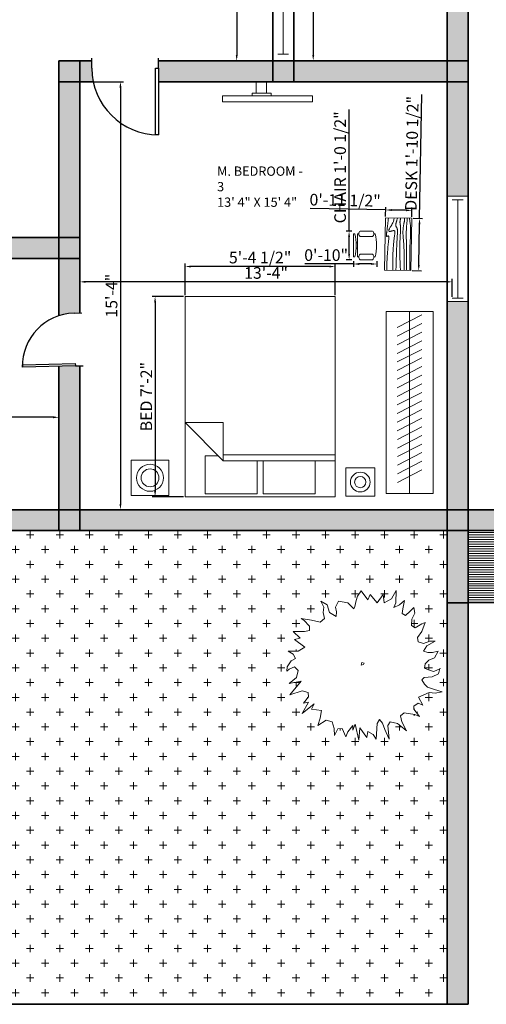
# Model space of a CAD drawing. Units: millimetres. Extents: x 2768 to 4359, y 795 to 1583.
# Tile 7 of 13: x 3880 to 4080, y 835 to 1258. Entities that reach past the tile are written whole.
import ezdxf

# ---------------------------------------------------------------- set-up
doc = ezdxf.new("R2010")
doc.units = ezdxf.units.MM
for name, color, linetype, lineweight in [('A-ANNO-DIMS', 90, 'Continuous', 18), ('A-AREA-IDEN', 190, 'Continuous', 18), ('A-DOOR-PATT', 251, 'Continuous', 13), ('A-EQPM', 50, 'Continuous', 18), ('A-FLOR-CASE', 50, 'Continuous', 18), ('A-FLOR-CASE-PATT', 50, 'Continuous', 13), ('A-WALL-PATT', 140, 'Continuous', 9), ('doors', 10, 'Continuous', 25), ('furniture', 50, 'Continuous', 18), ('GARDEN', 109, 'Continuous', 18), ('iron shutter', 251, 'Continuous', 18), ('L-PLNT-PATT', 109, 'Continuous', 13), ('walls', 140, 'Continuous', 35), ('windows', 30, 'Continuous', 18)]:
    doc.layers.add(name, color=color, linetype=linetype, lineweight=lineweight)
doc.styles.get("Standard").update_dxf_attribs({"font": 'arial.ttf'})
doc.dimstyles.new('ISO-25', dxfattribs={"dimtxt": 5, "dimasz": 2.5, "dimexe": 1.25, "dimexo": 0.625, "dimtad": 1, "dimdec": 0, "dimlunit": 3, "dimtxsty": 'Standard', "dimcen": 2.5, "dimadec": 0, "dimazin": 0, "dimtfac": 1, "dimtdec": 0, "dimtmove": 0, "dimatfit": 3, "dimfxl": 1, "dimarcsym": 0})

# ---------------------------------------------------------------- blocks, each defined once
blk = doc.blocks.new('*U2')
for p, q in [((0, 0), (0, -6)), ((40, 0), (40, -6))]:
    blk.add_line(p, q)
blk.add_lwpolyline([(0, 0), (0, 40), (1.75, 40), (1.75, 0)], close=True)
blk.add_arc((0, 0), 40, 0, 90)
blk = doc.blocks.new('*U39')
for p, q in [((0, 4), (0, 0)), ((36, 4), (36, 0)), ((0, 2), (36, 2))]:
    blk.add_line(p, q)
blk = doc.blocks.new('Bed - Queen')
for p, q in [((0, -80.00003), (0, 0)), ((0, 0), (59.99999, 0)), ((59.99999, 0), (59.99999, -80.00003)), ((7.99999, -1.2), (28.79998, -1.2)), ((7.99999, -14.4), (7.99999, -1.2)), ((28.79998, -1.2), (28.79998, -14.4)), ((31.19999, -1.2), (51.99999, -1.2)), ((31.19999, -14.4), (31.19999, -1.2)), ((51.99999, -1.2), (51.99999, -16.4)), ((0, -14.4), (44.8, -14.4)), ((59.99999, -29.6), (44.8, -14.4)), ((44.8, -14.4), (44.8, -29.6)), ((44.8, -16.8), (0, -16.8)), ((51.99999, -16.4), (46.79936, -16.4)), ((44.8, -29.6), (59.99999, -29.6)), ((59.99999, -80.00003), (0, -80.00003))]:
    blk.add_line(p, q)
blk = doc.blocks.new('Table - Rectangular Woodgrain 60 x 30 in.')
for p, q in [((0, 0), (0, -30)), ((60, 0), (0, 0)), ((60, -30), (60, 0)), ((0, -30), (60, -30))]:
    blk.add_line(p, q)
for points in [[(0, -2.4), (4.8155, -2.418), (9.0302, -2.4688), (12.709, -2.5477), (15.9167, -2.65), (18.7181, -2.7711), (21.1781, -2.9063), (23.3616, -3.0508), (25.3333, -3.2), (27.1477, -3.3495), (28.8172, -3.4958), (30.3437, -3.636), (31.7291, -3.7667), (32.9756, -3.8849), (34.0849, -3.9875), (35.059, -4.0714), (35.9, -4.1334), (36.6114, -4.1711), (37.2041, -4.1854), (37.6906, -4.1779), (38.0833, -4.15), (38.3948, -4.1034), (38.6375, -4.0396), (38.8239, -3.9602), (38.9666, -3.8667), (39.0764, -3.7608), (39.1573, -3.6448), (39.2116, -3.521), (39.2416, -3.3917), (39.2498, -3.2593), (39.2385, -3.1261), (39.21, -2.9944), (39.1666, -2.8667), (39.111, -2.7447), (39.0468, -2.6281), (38.978, -2.5163), (38.9083, -2.4083), (38.8418, -2.3035), (38.7823, -2.201), (38.7337, -2.1001), (38.7, -2), (38.6844, -1.9003), (38.6875, -1.8021), (38.7094, -1.707), (38.75, -1.6167), (38.8094, -1.5326), (38.8875, -1.4563), (38.9844, -1.3893), (39.1, -1.3333), (39.2351, -1.2896), (39.3937, -1.2583), (39.5804, -1.2396), (39.8, -1.2333), (40.057, -1.2396), (40.3562, -1.2583), (40.7023, -1.2896), (41.1, -1.3333), (41.5547, -1.3895), (42.0755, -1.4573), (42.6721, -1.5361), (43.3542, -1.625), (44.1316, -1.7233), (45.014, -1.8302), (46.0114, -1.9449), (47.1333, -2.0667), (48.3862, -2.1947), (49.7625, -2.3281), (51.2513, -2.4663), (52.8416, -2.6083), (54.5226, -2.7535), (56.2833, -2.9011), (58.1127, -3.0501), (60, -3.2)], [(0, -9.2), (6.5759, -9.0858), (11.9385, -9.0365), (16.2527, -9.0418), (19.6833, -9.0917), (22.3952, -9.1759), (24.5531, -9.2844), (26.322, -9.4069), (27.8666, -9.5333), (29.3241, -9.6553), (30.7203, -9.7719), (32.0532, -9.8837), (33.3208, -9.9917), (34.5213, -10.0965), (35.6526, -10.199), (36.7128, -10.2999), (37.7, -10.4), (38.6129, -10.4996), (39.4531, -10.5969), (40.223, -10.6895), (40.925, -10.775), (41.5613, -10.8512), (42.1344, -10.9156), (42.6465, -10.966), (43.1, -11), (43.4976, -11.0158), (43.8437, -11.0136), (44.143, -10.9942), (44.4, -10.9583), (44.6195, -10.9069), (44.8062, -10.8406), (44.9648, -10.7603), (45.1, -10.6667), (45.2155, -10.5598), (45.3114, -10.4365), (45.3871, -10.2929), (45.4416, -10.125), (45.4743, -9.929), (45.4844, -9.7011), (45.4709, -9.4371), (45.4333, -9.1333), (45.3716, -8.7883), (45.2896, -8.4104), (45.1919, -8.0107), (45.0833, -7.6), (44.9685, -7.1893), (44.8521, -6.7896), (44.7388, -6.4117), (44.6333, -6.0667), (44.54, -5.7628), (44.4614, -5.4979), (44.4001, -5.2675), (44.3583, -5.0667), (44.3384, -4.8909), (44.3427, -4.7354), (44.3736, -4.5956), (44.4333, -4.4667), (44.5236, -4.3453), (44.6427, -4.2333), (44.7884, -4.1339), (44.9583, -4.05), (45.1501, -3.9849), (45.3614, -3.9417), (45.59, -3.9234), (45.8333, -3.9333), (46.0915, -3.9749), (46.3734, -4.0531), (46.6906, -4.1736), (47.0542, -4.3417), (47.4756, -4.5629), (47.9661, -4.8427), (48.5372, -5.1866), (49.2, -5.6), (49.9676, -6.0844), (50.8594, -6.625), (51.8965, -7.2031), (53.1, -7.8), (54.491, -8.3969), (56.0906, -8.975), (57.9199, -9.5156), (60, -10)], [(0, -12.8), (5.1847, -12.9322), (9.6213, -13.0323), (13.3963, -13.1059), (16.5958, -13.1583), (19.3063, -13.1952), (21.614, -13.2219), (23.6054, -13.2439), (25.3666, -13.2667), (26.9728, -13.2947), (28.4531, -13.3281), (29.8256, -13.3663), (31.1083, -13.4083), (32.3191, -13.4535), (33.476, -13.501), (34.597, -13.5501), (35.7, -13.6), (36.7984, -13.6497), (37.8875, -13.6979), (38.9578, -13.743), (40, -13.7833), (41.0047, -13.8174), (41.9625, -13.8438), (42.864, -13.8607), (43.7, -13.8667), (44.4631, -13.8604), (45.1552, -13.8417), (45.7801, -13.8104), (46.3416, -13.7667), (46.8439, -13.7104), (47.2906, -13.6417), (47.6858, -13.5604), (48.0333, -13.4667), (48.3375, -13.3608), (48.6042, -13.2448), (48.8396, -13.121), (49.05, -12.9917), (49.2417, -12.8593), (49.4208, -12.7261), (49.5937, -12.5944), (49.7667, -12.4667), (49.9452, -12.3451), (50.1323, -12.2313), (50.3303, -12.1268), (50.5416, -12.0333), (50.7686, -11.9524), (51.0135, -11.8854), (51.2788, -11.8341), (51.5666, -11.8), (51.8785, -11.7843), (52.2116, -11.7865), (52.562, -11.8059), (52.926, -11.8417), (53.2998, -11.8931), (53.6795, -11.9594), (54.0614, -12.0397), (54.4416, -12.1333), (54.8223, -12.2401), (55.2293, -12.3625), (55.6942, -12.5037), (56.2489, -12.6667), (56.9251, -12.8547), (57.7545, -13.0708), (58.7689, -13.3182), (60, -13.6)], [(0, -18), (5.124, -17.7273), (9.6609, -17.5057), (13.6705, -17.3303), (17.2125, -17.1958), (20.3467, -17.0973), (23.1328, -17.0297), (25.6307, -16.9878), (27.9, -16.9667), (29.9928, -16.9617), (31.9302, -16.9703), (33.7254, -16.9907), (35.3917, -17.0208), (36.9423, -17.0588), (38.3906, -17.1026), (39.7499, -17.1503), (41.0333, -17.2), (42.2519, -17.2496), (43.4073, -17.2969), (44.4986, -17.3395), (45.525, -17.375), (46.4858, -17.4012), (47.3802, -17.4156), (48.2074, -17.416), (48.9667, -17.4), (49.6583, -17.3662), (50.2872, -17.3167), (50.8595, -17.2547), (51.3812, -17.1833), (51.8584, -17.1057), (52.2971, -17.025), (52.7034, -16.9443), (53.0833, -16.8667), (53.443, -16.7951), (53.789, -16.7313), (54.128, -16.6768), (54.4666, -16.6334), (54.8115, -16.6024), (55.1693, -16.5854), (55.5465, -16.5841), (55.95, -16.6), (56.3828, -16.6337), (56.8346, -16.6823), (57.2915, -16.7418), (57.7396, -16.8084), (58.165, -16.878), (58.5539, -16.9469), (58.8924, -17.0111), (59.1666, -17.0667), (59.3679, -17.1107), (59.5078, -17.1438), (59.6032, -17.1675), (59.6708, -17.1833), (59.7275, -17.193), (59.7901, -17.1979), (59.8753, -17.1998), (60, -17.2)], [(0, -22.4), (8.0098, -22.2501), (14.4094, -22.1011), (19.4168, -21.9535), (23.25, -21.8083), (26.1269, -21.6663), (28.2656, -21.5281), (29.884, -21.3947), (31.2, -21.2667), (32.3967, -21.1448), (33.5172, -21.0292), (34.5697, -20.9198), (35.5625, -20.8167), (36.5037, -20.7198), (37.4015, -20.6292), (38.2642, -20.5448), (39.1, -20.4667), (39.9164, -20.3951), (40.7187, -20.3313), (41.5117, -20.2768), (42.3, -20.2333), (43.0883, -20.2024), (43.8812, -20.1854), (44.6836, -20.1841), (45.5, -20.2), (46.3328, -20.234), (47.1747, -20.2844), (48.0163, -20.3488), (48.8479, -20.425), (49.66, -20.5106), (50.4429, -20.6031), (51.1872, -20.7004), (51.8833, -20.8), (52.5246, -20.8999), (53.1166, -20.9995), (53.6681, -21.0983), (54.1875, -21.1958), (54.6834, -21.2919), (55.1646, -21.3859), (55.6394, -21.4777), (56.1167, -21.5667), (56.6028, -21.6515), (57.0961, -21.7266), (57.5929, -21.7852), (58.0896, -21.8208), (58.5823, -21.8268), (59.0674, -21.7964), (59.5412, -21.723), (60, -21.6)], [(0, -25.2), (8.6355, -25.0504), (15.7026, -24.9031), (21.4049, -24.7606), (25.9458, -24.625), (29.529, -24.4988), (32.3578, -24.3844), (34.6359, -24.284), (36.5667, -24.2), (38.3213, -24.1341), (39.9417, -24.0854), (41.437, -24.0523), (42.8167, -24.0333), (44.0901, -24.0268), (45.2667, -24.0313), (46.3557, -24.0451), (47.3667, -24.0667), (48.309, -24.0947), (49.1928, -24.1287), (50.0284, -24.168), (50.826, -24.2125), (51.5959, -24.2617), (52.3483, -24.3151), (53.0935, -24.3725), (53.8417, -24.4334), (54.6009, -24.497), (55.3699, -24.561), (56.1454, -24.6226), (56.9239, -24.6792), (57.7021, -24.7279), (58.4764, -24.7662), (59.2435, -24.7911), (60, -24.8)], [(0, -28.8), (5.6867, -28.6681), (10.45, -28.5698), (14.407, -28.5012), (17.675, -28.4584), (20.3711, -28.4374), (22.6125, -28.4344), (24.5164, -28.4455), (26.2, -28.4667), (27.762, -28.4947), (29.2276, -28.5281), (30.6033, -28.5663), (31.8958, -28.6084), (33.1118, -28.6535), (34.2578, -28.7011), (35.3405, -28.7501), (36.3666, -28.8), (37.3443, -28.8497), (38.288, -28.8974), (39.2137, -28.9412), (40.1375, -28.9792), (41.0753, -29.0093), (42.0432, -29.0297), (43.0572, -29.0384), (44.1333, -29.0333), (45.2936, -29.0114), (46.5843, -28.9641), (48.0579, -28.8816), (49.7666, -28.7542), (51.7629, -28.5721), (54.0989, -28.3255), (56.8272, -28.0048), (60, -27.6)]]:
    blk.add_lwpolyline(points)
blk = doc.blocks.new('Chair - Desk')
for p, q in [((-8.5, 0), (-8.5, -1)), ((-8.5, 0), (8.5, 0)), ((8.5, 0), (8.5, -1)), ((-10.5, -5), (-10.5, -14)), ((-8.5, -3), (-8.5, -4)), ((-8.5, -3), (8.5, -3)), ((-6.5, -14), (-6.5, -5)), ((-2, -3), (-2, -1.9355)), ((2, -1.9576), (2, -3)), ((6.5, -5), (6.5, -14)), ((8.5, -3), (8.5, -4)), ((10.5, -14), (10.5, -5)), ((-8.5, -15), (-8.5, -16)), ((8.5, -15), (8.5, -16))]:
    blk.add_line(p, q)
for centre, radius, start, end in [((-8.5, -6.5), 2.5, 36.8699, 143.1301), ((0, 34.625), 36.625, 256.5803, 283.4197), ((8.5, -6.5), 2.5, 36.8699, 143.1301), ((-8.5, -12.5), 2.5, 216.8699, 323.1301), ((8.5, -12.5), 2.5, 216.8699, 323.1301), ((0, 19.625), 36.625, 256.5803, 283.4197)]:
    blk.add_arc(centre, radius, start, end)
blk = doc.blocks.new('*D56')
at = {"layer": 'A-ANNO-DIMS', "color": 0, "lineweight": -2, "transparency": 16777216}
for p, q in [((3836.37, 1089), (3836.37, 1086.28)), ((3896.37, 1089), (3896.37, 1086.28)), ((3893.87, 1087.53), (3838.87, 1087.53))]:
    blk.add_line(p, q, dxfattribs=at)
at = {"layer": 'A-ANNO-DIMS', "color": 0, "transparency": 16777216}
for points in [[(3838.87, 1087.95), (3838.87, 1087.12), (3836.37, 1087.53)], [(3893.87, 1087.95), (3893.87, 1087.12), (3896.37, 1087.53)]]:
    blk.add_solid(points, dxfattribs=at)
at = {"layer": 'Defpoints', "color": 0, "transparency": 16777216}
for p in [(3836.37, 1089.62), (3896.37, 1089.62), (3836.37, 1087.53)]:
    blk.add_point(p, dxfattribs=at)
at = {"layer": 'A-ANNO-DIMS', "color": 0, "transparency": 16777216, "insert": (3866.37, 1090.7), "char_height": 5, "attachment_point": 5}
blk.add_mtext("5'", dxfattribs=at)
blk = doc.blocks.new('*D57')
at = {"layer": 'A-ANNO-DIMS', "color": 0, "lineweight": -2, "transparency": 16777216}
for p, q in [((3905.37, 1139.32), (3905.37, 1147.01)), ((4063.11, 1145.76), (3907.87, 1145.76)), ((4065.61, 1139.32), (4065.61, 1147.01))]:
    blk.add_line(p, q, dxfattribs=at)
at = {"layer": 'A-ANNO-DIMS', "color": 0, "transparency": 16777216}
for points in [[(3907.87, 1146.18), (3907.87, 1145.34), (3905.37, 1145.76)], [(4063.11, 1146.18), (4063.11, 1145.34), (4065.61, 1145.76)]]:
    blk.add_solid(points, dxfattribs=at)
at = {"layer": 'Defpoints', "color": 0, "transparency": 16777216}
for p in [(3905.37, 1145.76), (3905.37, 1138.7), (4065.61, 1138.7)]:
    blk.add_point(p, dxfattribs=at)
at = {"layer": 'A-ANNO-DIMS', "color": 0, "transparency": 16777216, "insert": (3985.49, 1148.94), "char_height": 5, "attachment_point": 5}
blk.add_mtext('13\'-4"', dxfattribs=at)
blk = doc.blocks.new('*D58')
at = {"layer": 'A-ANNO-DIMS', "color": 0, "lineweight": -2, "transparency": 16777216}
for p, q in [((3908.8, 1231.81), (3924.1, 1231.81)), ((3922.85, 1229.31), (3922.85, 1050.31)), ((3908.8, 1047.81), (3924.1, 1047.81))]:
    blk.add_line(p, q, dxfattribs=at)
at = {"layer": 'A-ANNO-DIMS', "color": 0, "transparency": 16777216}
for points in [[(3922.44, 1229.31), (3923.27, 1229.31), (3922.85, 1231.81)], [(3922.44, 1050.31), (3923.27, 1050.31), (3922.85, 1047.81)]]:
    blk.add_solid(points, dxfattribs=at)
at = {"layer": 'Defpoints', "color": 0, "transparency": 16777216}
for p in [(3908.17, 1231.81), (3908.17, 1047.81), (3922.85, 1047.81)]:
    blk.add_point(p, dxfattribs=at)
at = {"layer": 'A-ANNO-DIMS', "color": 0, "transparency": 16777216, "insert": (3919.68, 1139.81), "char_height": 5, "attachment_point": 5, "rotation": 90}
blk.add_mtext('15\'-4"', dxfattribs=at)
blk = doc.blocks.new('*D61')
at = {"layer": 'A-ANNO-DIMS', "color": 0, "lineweight": -2, "transparency": 16777216}
for p, q in [((4003.77, 1378.81), (4007.03, 1378.81)), ((4005.78, 1376.31), (4005.78, 1243.31)), ((4003.77, 1240.81), (4007.03, 1240.81))]:
    blk.add_line(p, q, dxfattribs=at)
at = {"layer": 'A-ANNO-DIMS', "color": 0, "transparency": 16777216}
for points in [[(4005.36, 1376.31), (4006.2, 1376.31), (4005.78, 1378.81)], [(4005.36, 1243.31), (4006.2, 1243.31), (4005.78, 1240.81)]]:
    blk.add_solid(points, dxfattribs=at)
at = {"layer": 'Defpoints', "color": 0, "transparency": 16777216}
for p in [(4003.15, 1378.81), (4003.15, 1240.81), (4005.78, 1240.81)]:
    blk.add_point(p, dxfattribs=at)
at = {"layer": 'A-ANNO-DIMS', "color": 0, "transparency": 16777216, "insert": (4002.6, 1309.81), "char_height": 5, "attachment_point": 5, "rotation": 90}
blk.add_mtext('11\'-6"', dxfattribs=at)
blk = doc.blocks.new('*D62')
at = {"layer": 'A-ANNO-DIMS', "color": 0, "lineweight": -2, "transparency": 16777216}
for p, q in [((3972.05, 1378.81), (3974.11, 1378.81)), ((3972.86, 1376.31), (3972.86, 1243.31)), ((3972.05, 1240.81), (3974.11, 1240.81))]:
    blk.add_line(p, q, dxfattribs=at)
at = {"layer": 'A-ANNO-DIMS', "color": 0, "transparency": 16777216}
for points in [[(3972.45, 1376.31), (3973.28, 1376.31), (3972.86, 1378.81)], [(3972.45, 1243.31), (3973.28, 1243.31), (3972.86, 1240.81)]]:
    blk.add_solid(points, dxfattribs=at)
at = {"layer": 'Defpoints', "color": 0, "transparency": 16777216}
for p in [(3971.42, 1378.81), (3971.42, 1240.81), (3972.86, 1240.81)]:
    blk.add_point(p, dxfattribs=at)
at = {"layer": 'A-ANNO-DIMS', "color": 0, "transparency": 16777216, "insert": (3969.69, 1309.81), "char_height": 5, "attachment_point": 5, "rotation": 90}
blk.add_mtext('11\'-6"', dxfattribs=at)
blk = doc.blocks.new('*U72')
for points in [[(0, 60.64), (-3.051, 56.238), (-4.196, 52.815), (-5.34, 47.925), (-6.103, 45.969), (-11.062, 50.859), (-18.691, 52.326), (-20.98, 47.436), (-20.217, 43.524), (-20.598, 39.611), (-25.939, 43.035), (-27.846, 49.392), (-33.186, 52.326), (-30.516, 47.436), (-31.279, 43.035), (-30.135, 38.144), (-33.568, 35.21), (-40.815, 36.677), (-49.208, 38.144), (-46.919, 36.677), (-42.341, 31.787), (-42.341, 28.364), (-46.537, 27.386), (-55.692, 27.386), (-49.97, 22.006), (-54.548, 21.028), (-46.156, 14.671), (-51.496, 11.248), (-59.888, 11.248), (-55.692, 8.803), (-53.785, 5.38), (-57.218, 3.423), (-60.651, -1.467), (-61.033, -4.89), (-59.125, -3.423), (-54.548, -1.467), (-51.496, -4.401), (-53.022, -10.269), (-59.125, -15.16), (-49.208, -13.204), (-58.362, -24.451), (-48.445, -21.028), (-43.486, -22.495), (-43.104, -25.918), (-47.3, -31.298), (-43.104, -30.32), (-48.445, -39.611), (-38.527, -31.787), (-40.815, -36.188), (-32.423, -37.166), (-33.568, -43.523), (-35.475, -49.392), (-28.609, -44.99), (-23.65, -46.457), (-22.124, -51.837), (-21.743, -57.705), (-19.073, -52.326), (-15.639, -51.837), (-12.588, -58.683), (-11.062, -54.771), (-6.866, -49.392), (-6.866, -53.304), (-4.959, -48.414), (-1.907, -61.617), (-1.144, -51.348), (4.578, -59.172), (5.341, -54.282), (9.918, -56.727), (12.207, -60.639), (12.97, -47.925), (14.877, -44.501), (17.547, -47.436), (19.455, -52.815), (22.888, -60.639), (21.743, -49.392), (23.65, -46.457), (29.754, -47.925), (35.094, -52.326), (37.001, -53.793), (33.187, -46.457), (32.042, -41.567), (35.094, -39.122), (43.868, -40.589), (47.682, -42.056), (43.105, -36.188), (43.105, -33.743), (46.538, -31.298), (50.352, -32.765), (46.919, -26.407), (55.693, -22.495), (60.652, -22.984), (66.374, -22.006), (59.889, -20.05), (54.167, -18.094), (51.878, -15.649), (49.589, -12.225), (51.497, -10.269), (57.981, -9.78), (63.322, -7.335), (64.466, -2.934)], [(64.848, -2.934), (59.507, -5.379), (56.456, -4.401), (51.878, -2.445), (52.26, 0.978), (55.311, 3.912), (59.889, 5.869), (62.94, 11.248), (58.363, 10.27), (54.548, 10.27), (51.115, 11.248), (53.785, 15.649), (57.981, 18.094), (60.652, 19.561), (56.074, 19.561), (51.115, 17.605), (46.538, 19.072), (46.156, 22.496), (49.589, 27.386), (52.26, 34.721), (49.589, 33.743), (44.249, 30.32), (41.197, 32.276), (41.579, 37.655), (43.868, 42.546), (43.105, 46.947), (40.053, 44.013), (36.238, 40.589), (33.568, 42.057), (33.95, 45.969), (35.476, 52.815), (31.28, 49.392), (26.702, 46.947), (28.228, 50.859), (28.609, 61.129), (24.795, 54.282), (18.692, 50.859), (17.929, 57.706), (12.97, 50.859), (7.248, 57.706), (5.341, 53.304), (0, 60.64)]]:
    blk.add_lwpolyline(points)
blk.add_lwpolyline([(0.382, 1.956), (0, 0), (1.907, 0.489), (2.289, 1.467)], close=True)
blk = doc.blocks.new('*D91')
at = {"layer": 'A-ANNO-DIMS', "color": 0, "lineweight": -2, "transparency": 16777216}
for p, q in [((4021.21, 1167.59), (4021.21, 1219.89)), ((4022.43, 1167.59), (4019.96, 1167.59)), ((4021.21, 1157.78), (4021.21, 1165.09)), ((4022.43, 1155.28), (4019.96, 1155.28))]:
    blk.add_line(p, q, dxfattribs=at)
at = {"layer": 'A-ANNO-DIMS', "color": 0, "transparency": 16777216}
for points in [[(4020.79, 1165.09), (4021.62, 1165.09), (4021.21, 1167.59)], [(4020.79, 1157.78), (4021.62, 1157.78), (4021.21, 1155.28)]]:
    blk.add_solid(points, dxfattribs=at)
at = {"layer": 'Defpoints', "color": 0, "transparency": 16777216}
for p in [(4021.21, 1167.59), (4023.05, 1167.59), (4023.05, 1155.28)]:
    blk.add_point(p, dxfattribs=at)
at = {"layer": 'A-ANNO-DIMS', "color": 0, "transparency": 16777216, "insert": (4018, 1194.99), "char_height": 5, "attachment_point": 5, "rotation": 90}
blk.add_mtext('CHAIR 1\'-0 1/2"', dxfattribs=at)
blk = doc.blocks.new('*D92')
at = {"layer": 'A-ANNO-DIMS', "color": 0, "lineweight": -2, "transparency": 16777216}
for p, q in [((4023.05, 1153.44), (4002.13, 1153.44)), ((4023.05, 1154.66), (4023.05, 1152.19)), ((4030.71, 1153.44), (4025.55, 1153.44)), ((4033.21, 1154.66), (4033.21, 1152.19))]:
    blk.add_line(p, q, dxfattribs=at)
at = {"layer": 'A-ANNO-DIMS', "color": 0, "transparency": 16777216}
for points in [[(4025.55, 1153.85), (4025.55, 1153.02), (4023.05, 1153.44)], [(4030.71, 1153.85), (4030.71, 1153.02), (4033.21, 1153.44)]]:
    blk.add_solid(points, dxfattribs=at)
at = {"layer": 'Defpoints', "color": 0, "transparency": 16777216}
for p in [(4023.05, 1155.28), (4023.05, 1153.44), (4033.21, 1155.28)]:
    blk.add_point(p, dxfattribs=at)
at = {"layer": 'A-ANNO-DIMS', "color": 0, "transparency": 16777216, "insert": (4011.34, 1156.61), "char_height": 5, "attachment_point": 5}
blk.add_mtext('0\'-10"', dxfattribs=at)
blk = doc.blocks.new('*D99')
at = {"layer": 'A-ANNO-DIMS', "color": 0, "lineweight": -2, "transparency": 16777216}
for p, q in [((3950.04, 1139.44), (3936.51, 1139.44)), ((3937.76, 1136.94), (3937.76, 1055.89)), ((3950.04, 1053.39), (3936.51, 1053.39))]:
    blk.add_line(p, q, dxfattribs=at)
at = {"layer": 'A-ANNO-DIMS', "color": 0, "transparency": 16777216}
for points in [[(3937.34, 1136.94), (3938.18, 1136.94), (3937.76, 1139.44)], [(3937.34, 1055.89), (3938.18, 1055.89), (3937.76, 1053.39)]]:
    blk.add_solid(points, dxfattribs=at)
at = {"layer": 'Defpoints', "color": 0, "transparency": 16777216}
for p in [(3950.67, 1139.44), (3937.76, 1053.39), (3950.67, 1053.39)]:
    blk.add_point(p, dxfattribs=at)
at = {"layer": 'A-ANNO-DIMS', "color": 0, "transparency": 16777216, "insert": (3934.62, 1096.42), "char_height": 5, "attachment_point": 5, "rotation": 90}
blk.add_mtext('BED 7\'-2"', dxfattribs=at)
blk = doc.blocks.new('*D100')
at = {"layer": 'A-ANNO-DIMS', "color": 0, "lineweight": -2, "transparency": 16777216}
for p, q in [((3950.67, 1140.07), (3950.67, 1153.6)), ((4012.7, 1152.35), (3953.17, 1152.35)), ((4015.2, 1140.07), (4015.2, 1153.6))]:
    blk.add_line(p, q, dxfattribs=at)
at = {"layer": 'A-ANNO-DIMS', "color": 0, "transparency": 16777216}
for points in [[(3953.17, 1152.77), (3953.17, 1151.93), (3950.67, 1152.35)], [(4012.7, 1152.77), (4012.7, 1151.93), (4015.2, 1152.35)]]:
    blk.add_solid(points, dxfattribs=at)
at = {"layer": 'Defpoints', "color": 0, "transparency": 16777216}
for p in [(3950.67, 1152.35), (3950.67, 1139.44), (4015.2, 1139.44)]:
    blk.add_point(p, dxfattribs=at)
at = {"layer": 'A-ANNO-DIMS', "color": 0, "transparency": 16777216, "insert": (3982.94, 1155.56), "char_height": 5, "attachment_point": 5}
blk.add_mtext('5\'-4 1/2"', dxfattribs=at)
blk = doc.blocks.new('*D115')
at = {"layer": 'A-ANNO-DIMS', "color": 0, "lineweight": -2, "transparency": 16777216}
for p, q in [((4051.54, 1173.03), (4052.5, 1226.31)), ((4048.79, 1173.08), (4052.79, 1173.01)), ((4051.18, 1153.02), (4051.5, 1170.53)), ((4048.38, 1150.57), (4052.39, 1150.5))]:
    blk.add_line(p, q, dxfattribs=at)
at = {"layer": 'A-ANNO-DIMS', "color": 0, "transparency": 16777216}
for points in [[(4051.08, 1170.54), (4051.91, 1170.52), (4051.54, 1173.03)], [(4050.76, 1153.03), (4051.6, 1153.01), (4051.14, 1150.52)]]:
    blk.add_solid(points, dxfattribs=at)
at = {"layer": 'Defpoints', "color": 0, "transparency": 16777216}
for p in [(4048.17, 1173.09), (4051.54, 1173.03), (4047.76, 1150.58)]:
    blk.add_point(p, dxfattribs=at)
at = {"layer": 'A-ANNO-DIMS', "color": 0, "transparency": 16777216, "insert": (4048.84, 1200.98), "char_height": 5, "attachment_point": 5, "rotation": 88.9651}
blk.add_mtext('DESK 1\'-10 1/2"', dxfattribs=at)
blk = doc.blocks.new('*D116')
at = {"layer": 'A-ANNO-DIMS', "color": 0, "lineweight": -2, "transparency": 16777216}
for p, q in [((4036.97, 1176.67), (4004.4, 1177.26)), ((4036.92, 1173.92), (4036.99, 1177.92)), ((4048.18, 1173.72), (4048.25, 1177.72)), ((4045.73, 1176.51), (4039.47, 1176.62))]:
    blk.add_line(p, q, dxfattribs=at)
at = {"layer": 'A-ANNO-DIMS', "color": 0, "transparency": 16777216}
for points in [[(4039.48, 1177.04), (4039.46, 1176.21), (4036.97, 1176.67)], [(4045.73, 1176.93), (4045.72, 1176.1), (4048.23, 1176.47)]]:
    blk.add_solid(points, dxfattribs=at)
at = {"layer": 'Defpoints', "color": 0, "transparency": 16777216}
for p in [(4036.91, 1173.29), (4036.97, 1176.67), (4048.17, 1173.09)]:
    blk.add_point(p, dxfattribs=at)
at = {"layer": 'A-ANNO-DIMS', "color": 0, "transparency": 16777216, "insert": (4019.49, 1180.2), "char_height": 5, "attachment_point": 5, "rotation": 358.9651}
blk.add_mtext('0\'-11 1/2"', dxfattribs=at)

msp = doc.modelspace()

# ---------------------------------------------------------------- hatches: boundary and pattern name
at = {"layer": 'A-DOOR-PATT'}
h = msp.add_hatch(dxfattribs=at)
h.set_pattern_fill('ANSI31', color=256, scale=0.3149606, angle=-45, style=0)
h.paths.add_polyline_path([(4072.37, 1038.81), (4313.37, 1038.81), (4313.37, 1007.81), (4072.37, 1007.81)])
at = {"layer": 'A-FLOR-CASE-PATT'}
h = msp.add_hatch(dxfattribs=at)
h.set_pattern_fill('ANSI31', color=256, scale=1.036594, angle=-17.802, style=0)
h.paths.add_polyline_path([(4052.51, 1062.35), (4041.97, 1056.93), (4041.93, 1127.22), (4052.48, 1132.64)])
at = {"layer": 'A-WALL-PATT'}
h = msp.add_hatch(color=256, dxfattribs=at)
h.dxf.hatch_style = 1
h.paths.add_polyline_path([(3666.8, 1540.81), (3628.37, 1540.81), (3628.37, 1531.81), (3666.8, 1531.81)])
h.paths.add_polyline_path([(3628.37, 1540.81), (3619.37, 1540.81), (3619.37, 1531.81), (3628.37, 1531.81)])
h.paths.add_polyline_path([(3628.37, 1531.81), (3619.37, 1531.81), (3619.37, 1387.81), (3628.37, 1387.81)])
h.paths.add_polyline_path([(3772.37, 1540.81), (3710.62, 1540.81), (3710.62, 1531.81), (3772.37, 1531.81)])
h.paths.add_polyline_path([(3796.31, 1540.81), (3781.37, 1540.81), (3781.37, 1531.81), (3796.31, 1531.81)])
h.paths.add_polyline_path([(3781.37, 1540.81), (3772.37, 1540.81), (3772.37, 1531.81), (3781.37, 1531.81)])
h.paths.add_polyline_path([(3781.37, 1531.81), (3772.37, 1531.81), (3772.37, 1493.05), (3773.51, 1493.08), (3781.37, 1493.27)])
h.paths.add_polyline_path([(3841.37, 1540.81), (3822.12, 1540.81), (3822.12, 1531.81), (3841.37, 1531.81)])
h.paths.add_polyline_path([(3867.29, 1540.81), (3850.37, 1540.81), (3850.37, 1531.81), (3867.29, 1531.81)])
h.paths.add_polyline_path([(3850.37, 1540.81), (3841.37, 1540.81), (3841.37, 1531.81), (3850.37, 1531.81)])
h.paths.add_polyline_path([(3850.37, 1531.81), (3841.37, 1531.81), (3841.37, 1435.81), (3850.37, 1435.81)])
h.paths.add_polyline_path([(3919.37, 1531.81), (3910.37, 1531.81), (3910.37, 1495.39, -0.097322), (3918.93, 1497.3), (3919.37, 1497.31)])
h.paths.add_polyline_path([(3919.37, 1540.81), (3910.37, 1540.81), (3910.37, 1531.81), (3919.37, 1531.81)])
h.paths.add_polyline_path([(3910.37, 1540.81), (3893.19, 1540.81), (3893.19, 1531.81), (3910.37, 1531.81)])
h.paths.add_polyline_path([(3971.85, 1540.81), (3919.37, 1540.81), (3919.37, 1531.81), (3971.85, 1531.81)])
h.paths.add_polyline_path([(4063.37, 1540.81), (4017.44, 1540.81), (4017.44, 1531.81), (4063.37, 1531.81)])
h.paths.add_polyline_path([(4072.37, 1531.81), (4063.37, 1531.81), (4063.37, 1387.81), (4072.37, 1387.81)])
h.paths.add_polyline_path([(4072.37, 1378.81), (4063.37, 1378.81), (4063.37, 1240.81), (4072.37, 1240.81)])
h.paths.add_polyline_path([(4072.37, 1387.81), (4063.37, 1387.81), (4063.37, 1378.81), (4072.37, 1378.81)])
h.paths.add_polyline_path([(3919.37, 1387.81), (3910.37, 1387.81), (3910.37, 1378.81), (3919.37, 1378.81)])
h.paths.add_polyline_path([(3919.37, 1392.95, -0.05459), (3913.18, 1392.28), (3910.37, 1392.28), (3910.37, 1387.81), (3919.37, 1387.81)])
h.paths.add_polyline_path([(3919.37, 1474.55), (3910.37, 1474.32), (3910.37, 1435.81), (3919.37, 1435.81)])
h.paths.add_polyline_path([(3919.37, 1435.81), (3910.37, 1435.81), (3910.37, 1426.81), (3919.37, 1426.81)])
h.paths.add_polyline_path([(3910.37, 1435.81), (3850.37, 1435.81), (3850.37, 1426.81), (3910.37, 1426.81)])
h.paths.add_polyline_path([(3919.37, 1426.81), (3910.37, 1426.81), (3910.37, 1420.86), (3913.18, 1420.86), (3919.37, 1420.86)])
h.paths.add_polyline_path([(3850.37, 1435.81), (3841.37, 1435.81), (3841.37, 1426.81), (3850.37, 1426.81)])
h.paths.add_polyline_path([(3841.37, 1435.81), (3781.37, 1435.81), (3781.37, 1426.81), (3841.37, 1426.81)])
h.paths.add_polyline_path([(3781.37, 1435.81), (3772.37, 1435.81), (3772.37, 1426.81), (3781.37, 1426.81)])
h.paths.add_polyline_path([(3781.37, 1426.81), (3772.37, 1426.81), (3772.37, 1420.59, -0.050492), (3778.09, 1421.17), (3781.37, 1421.17)])
h.paths.add_polyline_path([(3781.37, 1471.72, -0.082137), (3774.07, 1470.33), (3772.37, 1470.29), (3772.37, 1435.81), (3781.37, 1435.81)])
h.paths.add_polyline_path([(3628.37, 1387.81), (3619.37, 1387.81), (3619.37, 1378.81), (3628.37, 1378.81)])
h.paths.add_polyline_path([(3628.37, 1378.81), (3619.37, 1378.81), (3619.37, 1346.39), (3622.95, 1346.39), (3628.37, 1346.39)])
h.paths.add_polyline_path([(3781.37, 1387.81), (3772.37, 1387.81), (3772.37, 1378.81), (3781.37, 1378.81)])
h.paths.add_polyline_path([(3781.37, 1392.59), (3778.09, 1392.59), (3772.37, 1392.59), (3772.37, 1387.81), (3781.37, 1387.81)])
h.paths.add_polyline_path([(3628.37, 1318.32, -0.047705), (3622.95, 1317.81), (3619.37, 1317.81), (3619.37, 1221.81), (3628.37, 1221.81)])
h.paths.add_polyline_path([(3628.37, 1221.81), (3619.37, 1221.81), (3619.37, 1212.81), (3628.37, 1212.81)])
h.paths.add_polyline_path([(3827.37, 1221.81), (3628.37, 1221.81), (3628.37, 1212.81), (3827.37, 1212.81)])
h.paths.add_polyline_path([(3628.37, 1212.81), (3619.37, 1212.81), (3619.37, 1116.81), (3628.37, 1116.81)])
h.paths.add_polyline_path([(3836.37, 1221.81), (3827.37, 1221.81), (3827.37, 1212.81), (3836.37, 1212.81)])
h.paths.add_polyline_path([(3628.37, 1107.81), (3619.37, 1107.81), (3619.37, 1047.81), (3628.37, 1047.81)])
h.paths.add_polyline_path([(3628.37, 1116.81), (3619.37, 1116.81), (3619.37, 1107.81), (3628.37, 1107.81)])
h.paths.add_polyline_path([(3836.37, 1155.81), (3827.37, 1155.81), (3827.37, 1116.81), (3836.37, 1116.81)])
h.paths.add_polyline_path([(3836.37, 1116.81), (3827.37, 1116.81), (3827.37, 1107.81), (3836.37, 1107.81)])
h.paths.add_polyline_path([(3836.37, 1107.81), (3827.37, 1107.81), (3827.37, 1047.81), (3836.37, 1047.81)])
h.paths.add_polyline_path([(3827.37, 1047.37), (3827.37, 1047.81), (3739.96, 1047.81), (3739.96, 1038.81), (3827.37, 1038.81)])
h.paths.add_polyline_path([(3836.37, 1047.37), (3836.37, 1047.81), (3827.37, 1047.81), (3827.37, 1047.37), (3827.37, 1038.81), (3836.37, 1038.81)])
h.paths.add_polyline_path([(3695.08, 1047.81), (3628.37, 1047.81), (3628.37, 1038.81), (3695.08, 1038.81)])
h.paths.add_polyline_path([(3628.37, 1047.81), (3619.37, 1047.81), (3619.37, 1038.81), (3628.37, 1038.81)])
h.paths.add_polyline_path([(3850.59, 1047.81), (3836.37, 1047.81), (3836.37, 1047.37), (3836.37, 1038.81), (3850.59, 1038.81)])
h.paths.add_polyline_path([(3896.37, 1047.37), (3896.37, 1047.81), (3876.26, 1047.81), (3876.26, 1038.81), (3896.37, 1038.81)])
h.paths.add_polyline_path([(3905.37, 1109.65), (3903.46, 1109.6), (3896.37, 1109.43), (3896.37, 1047.81), (3905.37, 1047.81)])
h.paths.add_polyline_path([(3905.37, 1047.81), (3896.37, 1047.81), (3896.37, 1047.37), (3896.37, 1038.81), (3905.37, 1038.81)])
h.paths.add_polyline_path([(4063.37, 1047.81), (3905.37, 1047.81), (3905.37, 1038.81), (4063.37, 1038.81)])
h.paths.add_polyline_path([(4072.37, 1137.28), (4063.37, 1137.28), (4063.37, 1047.81), (4072.37, 1047.81)])
h.paths.add_polyline_path([(4072.37, 1231.81), (4063.37, 1231.81), (4063.37, 1182.55), (4072.37, 1182.55)])
h.paths.add_polyline_path([(4072.37, 1240.81), (4063.37, 1240.81), (4063.37, 1231.81), (4072.37, 1231.81)])
h.paths.add_polyline_path([(4072.37, 1047.81), (4063.37, 1047.81), (4063.37, 1038.81), (4072.37, 1038.81)])
h.paths.add_polyline_path([(3905.37, 1231.81), (3896.37, 1231.81), (3896.37, 1164.81), (3905.37, 1164.81)])
h.paths.add_polyline_path([(3905.37, 1240.81), (3896.37, 1240.81), (3896.37, 1231.81), (3905.37, 1231.81)])
h.paths.add_polyline_path([(3910.61, 1237.57), (3910.61, 1240.81), (3905.37, 1240.81), (3905.37, 1231.81), (3911.2, 1231.81, -0.050754)])
h.paths.add_polyline_path([(3988.37, 1240.81), (3939.19, 1240.81), (3939.19, 1237.57), (3939.19, 1231.81), (3988.37, 1231.81)])
h.paths.add_polyline_path([(3997.37, 1240.81), (3988.37, 1240.81), (3988.37, 1231.81), (3997.37, 1231.81)])
h.paths.add_polyline_path([(4063.37, 1240.81), (3997.37, 1240.81), (3997.37, 1231.81), (4063.37, 1231.81)])
h.paths.add_polyline_path([(3997.37, 1334.21), (3988.37, 1334.21), (3988.37, 1288.44), (3997.37, 1288.44)])
h.paths.add_polyline_path([(3896.37, 1164.81), (3836.37, 1164.81), (3836.37, 1155.81), (3896.37, 1155.81)])
h.paths.add_polyline_path([(3836.37, 1164.81), (3827.37, 1164.81), (3827.37, 1155.81), (3836.37, 1155.81)])
h.paths.add_polyline_path([(3905.37, 1164.81), (3896.37, 1164.81), (3896.37, 1155.81), (3905.37, 1155.81)])
h.paths.add_polyline_path([(3905.37, 1155.81), (3896.37, 1155.81), (3896.37, 1131.22, -0.073168), (3902.89, 1132.35), (3905.37, 1132.41)])
edge = h.paths.add_edge_path()
edge.add_line((3951.89, 1380.74), (3951.89, 1378.81))
edge.add_line((3951.89, 1378.81), (4063.37, 1378.81))
edge.add_line((4063.37, 1378.81), (4063.37, 1387.81))
edge.add_line((4063.37, 1387.81), (3951, 1387.81))
edge.add_arc((3923.31, 1380.74), 28.58, 0, 14.3236, ccw=False)
h.paths.add_polyline_path([(3923.31, 1378.81), (3923.31, 1387.81), (3919.37, 1387.81), (3919.37, 1378.81)])
edge = h.paths.add_edge_path()
edge.add_arc((3775.74, 1114.53), 22.75, 187.4686, 197.1843)
edge.add_line((3754, 1107.81), (3628.37, 1107.81))
edge.add_line((3628.37, 1107.81), (3628.37, 1116.81))
edge.add_line((3628.37, 1116.81), (3752.42, 1116.81))
edge.add_arc((3775.17, 1117.41), 22.75, 181.5276, 194.8757)
h.paths.add_polyline_path([(3775.68, 1116.81), (3775.91, 1107.81), (3827.37, 1107.81), (3827.37, 1116.81)])
h = msp.add_hatch(color=256, dxfattribs=at)
h.dxf.hatch_style = 1
h.paths.add_polyline_path([(4313.37, 1540.81), (4072.37, 1540.81), (4072.37, 1531.81), (4313.37, 1531.81)])
h.paths.add_polyline_path([(4072.37, 1540.81), (4063.37, 1540.81), (4063.37, 1531.81), (4072.37, 1531.81)])
h.paths.add_polyline_path([(4322.37, 1540.81), (4313.37, 1540.81), (4313.37, 1531.81), (4322.37, 1531.81)])
h.paths.add_polyline_path([(4322.37, 1531.81), (4313.37, 1531.81), (4313.37, 1378.81), (4313.37, 1047.81), (4322.37, 1047.81), (4322.37, 1378.81)])
h.paths.add_polyline_path([(4313.37, 1047.81), (4072.37, 1047.81), (4072.37, 1038.81), (4313.37, 1038.81)])
h = msp.add_hatch(color=256, dxfattribs=at)
h.dxf.hatch_style = 1
h.paths.add_polyline_path([(3628.37, 1038.81), (3619.37, 1038.81), (3619.37, 835.16), (3628.37, 835.16)])
h.paths.add_polyline_path([(4072.37, 1007.81), (4068.9, 1007.81), (4067.72, 1007.81), (4063.37, 1007.81), (4063.37, 835.16), (4072.37, 835.16)])
h = msp.add_hatch(color=256, dxfattribs=at)
h.dxf.hatch_style = 1
h.paths.add_polyline_path([(4063.37, 1007.81), (4067.72, 1007.81), (4068.9, 1007.81), (4072.37, 1007.81), (4072.37, 1038.81), (4063.37, 1038.81)])
at = {"layer": 'L-PLNT-PATT'}
h = msp.add_hatch(dxfattribs=at)
h.set_pattern_fill('CROSS', color=256)
h.set_pattern_definition([(0, (-194.219, 46.374), (6.35, 6.35), [3.175, -9.525]), (90, (-192.6314, 44.7867), (-6.35, 6.35), [3.175, -9.525])])
h.paths.add_polyline_path([(3628.37, 1038.81), (3628.37, 835.16), (4063.37, 835.16), (4063.37, 1007.81), (4063.37, 1038.81), (3905.37, 1038.81), (3896.37, 1038.81)])
h.paths.add_polyline_path([(3691.58, 971.77), (3691.54, 971.61), (3692.89, 969.92), (3693.09, 971.3)], flags=16)
h.paths.add_polyline_path([(3686.64, 970.14), (3687.8, 970.5), (3687.74, 971.09)], flags=16)
h.paths.add_polyline_path([(3726.85, 906.98), (3710.25, 904.9), (3713.35, 901.8), (3715.93, 901.89), (3726.61, 904.7, 0.029207)], flags=16)
h.paths.add_polyline_path([(3703.16, 924.71), (3703.15, 925.88), (3702.38, 925.11)], flags=16)
h.paths.add_polyline_path([(3994.35, 978.45), (3994.55, 980.25), (3996.36, 982.82), (3998.16, 983.85), (3997.16, 985.65), (3994.96, 986.93), (3999.36, 986.93), (4002.17, 988.73), (3997.76, 992.07), (4000.17, 992.58), (3997.16, 995.41), (4001.97, 995.41), (4004.17, 995.93), (4004.17, 997.72), (4001.77, 1000.29), (4000.57, 1001.06), (4004.98, 1000.29), (4008.78, 999.52), (4010.59, 1001.06), (4009.99, 1003.63), (4010.39, 1005.94), (4008.98, 1008.51), (4011.79, 1006.97), (4012.79, 1003.63), (4015.6, 1001.83), (4015.8, 1003.89), (4015.4, 1005.94), (4016.6, 1008.51), (4020.61, 1007.74), (4023.21, 1005.17), (4023.61, 1006.2), (4024.54, 1010.18), (4026.42, 1012.88), (4029.22, 1009.03), (4030.23, 1011.34), (4033.23, 1007.74), (4035.84, 1011.34), (4036.24, 1007.74), (4039.44, 1009.54), (4041.45, 1013.14), (4041.25, 1007.74), (4040.45, 1005.69), (4042.85, 1006.97), (4045.06, 1008.77), (4044.25, 1005.17), (4044.05, 1003.12), (4045.46, 1002.35), (4047.46, 1004.15), (4049.06, 1005.69), (4049.46, 1003.38), (4048.26, 1000.81), (4048.06, 997.98), (4049.66, 996.95), (4052.47, 998.75), (4053.87, 999.26), (4052.47, 995.41), (4050.67, 992.84), (4050.87, 991.04), (4053.27, 990.27), (4055.88, 991.3), (4058.28, 991.3), (4056.88, 990.53), (4054.67, 989.25), (4053.27, 986.93), (4055.08, 986.42), (4057.08, 986.42), (4059.48, 986.93), (4057.88, 984.11), (4055.48, 983.08), (4053.87, 981.54), (4053.67, 979.74), (4056.08, 978.71), (4057.68, 978.2), (4060.26, 979.38), (4059.68, 977.17), (4056.88, 975.89), (4053.47, 975.63), (4052.47, 974.6), (4053.67, 972.8), (4054.88, 971.52), (4057.88, 970.49), (4061.29, 969.46), (4058.28, 968.95), (4055.68, 969.21), (4051.07, 967.15), (4052.87, 963.81), (4050.87, 964.58), (4049.06, 963.3), (4049.06, 962.01), (4051.47, 958.93), (4049.46, 959.7), (4044.86, 960.47), (4043.25, 959.19), (4043.85, 956.62), (4045.86, 952.76), (4044.86, 953.53), (4042.05, 955.85), (4038.84, 956.62), (4037.84, 955.08), (4038.44, 949.17), (4036.64, 953.28), (4035.64, 956.1), (4034.23, 957.64), (4033.23, 955.85), (4032.83, 949.17), (4031.63, 951.22), (4029.22, 952.51), (4028.82, 949.94), (4025.82, 954.05), (4025.42, 948.65), (4023.81, 955.59), (4022.81, 953.02), (4022.81, 955.08), (4020.61, 952.25), (4019.81, 950.19), (4018.2, 953.79), (4016.4, 953.53), (4015, 950.71), (4014.8, 953.79), (4013.99, 956.62), (4011.39, 957.39), (4007.78, 955.08), (4008.78, 958.16), (4009.38, 961.5), (4004.98, 962.01), (4006.18, 964.32), (4000.97, 960.21), (4003.77, 965.1), (4001.57, 964.58), (4003.77, 967.41), (4003.57, 969.21), (4000.97, 969.98), (3995.76, 968.18), (4000.57, 974.09), (3995.36, 973.06), (3998.56, 975.63), (3999.36, 978.71), (3997.76, 980.25), (3995.36, 979.23)], flags=16)
h.paths.add_polyline_path([(4026.42, 981.02), (4026.62, 982.05), (4027.62, 981.79), (4027.42, 981.28)], flags=0)

# ---------------------------------------------------------------- linework, layer by layer
at = {"layer": 'A-EQPM'}
for p, q in [((3981.19, 1226.91), (3979.46, 1226.91)), ((3985.72, 1226.91), (3987.68, 1226.91))]:
    msp.add_line(p, q, dxfattribs=at)
for points in [[(3981.19, 1231.81), (3985.72, 1231.81), (3985.72, 1226.91), (3981.19, 1226.91)], [(3966.72, 1225.68), (4005.4, 1225.68), (4005.4, 1223.19), (3966.72, 1223.19)], [(3979.46, 1226.91), (3987.68, 1226.91), (3987.68, 1225.68), (3979.46, 1225.68)]]:
    msp.add_lwpolyline(points, close=True, dxfattribs=at)
at = {"layer": 'A-FLOR-CASE'}
msp.add_line((4047.2, 1133.01), (4047.2, 1054.76), dxfattribs=at)
msp.add_lwpolyline([(4057.3, 1054.76), (4037.1, 1054.76), (4037.1, 1133.01), (4057.3, 1133.01)], close=True, dxfattribs=at)
at = {"layer": 'furniture'}
for points in [[(3943.73, 1053.85), (3927.44, 1053.85), (3927.44, 1069.16), (3943.73, 1069.16)], [(4019.79, 1053.64), (4032.26, 1053.64), (4032.26, 1065.74), (4019.79, 1065.74)]]:
    msp.add_lwpolyline(points, close=True, dxfattribs=at)
for centre, radius in [((3935.59, 1061.51), 5.8), ((3935.59, 1061.51), 3.84), ((4026.03, 1059.69), 4.24), ((4026.03, 1059.69), 2.44)]:
    msp.add_circle(centre, radius, dxfattribs=at)
at = {"layer": 'iron shutter'}
for p, q in [((4072.37, 1038.81), (4313.37, 1038.81)), ((4072.37, 1007.81), (4313.37, 1007.81))]:
    msp.add_line(p, q, dxfattribs=at)
at = {"layer": 'walls'}
for p, q in [((3988.37, 1378.81), (3988.37, 1231.81)), ((3997.37, 1378.81), (3997.37, 1231.81)), ((4063.37, 1378.81), (4063.37, 1007.81)), ((4072.37, 1378.81), (4072.37, 1007.81)), ((3896.37, 1240.81), (3910.61, 1240.81)), ((3896.37, 1240.81), (3896.37, 1131.22)), ((3905.37, 1240.81), (3905.37, 1132.41)), ((3939.19, 1240.81), (4072.37, 1240.81)), ((3896.37, 1231.81), (3911.2, 1231.81)), ((3939.19, 1231.81), (4072.37, 1231.81)), ((3905.37, 1164.81), (3827.37, 1164.81)), ((3905.37, 1155.81), (3827.37, 1155.81)), ((3896.37, 1109.43), (3896.37, 1047.37)), ((3905.37, 1109.65), (3905.37, 1038.81)), ((3896.37, 1047.81), (3619.37, 1047.81)), ((3896.37, 1047.81), (4322.37, 1047.81)), ((3896.37, 1047.37), (3896.37, 1038.81)), ((3896.37, 1038.81), (3619.37, 1038.81)), ((3896.37, 1038.81), (3905.37, 1038.81)), ((3905.37, 1038.81), (4313.37, 1038.81)), ((4067.72, 1007.81), (4063.37, 1007.81)), ((4063.37, 1007.81), (4063.37, 835.16)), ((4068.9, 1007.81), (4067.72, 1007.81)), ((4072.37, 1007.81), (4068.9, 1007.81)), ((4072.37, 1007.81), (4072.37, 835.16)), ((4072.37, 835.16), (3619.37, 835.16))]:
    msp.add_line(p, q, dxfattribs=at)
at = {"layer": 'windows'}
for p, q in [((4072.37, 1182.55), (4063.37, 1182.55)), ((4072.37, 1137.28), (4063.37, 1137.28))]:
    msp.add_line(p, q, dxfattribs=at)

# ---------------------------------------------------------------- block references
at = {"layer": 'doors'}
for p, xscale, yscale, zscale, rotation in [((3939.19, 1237.57), 0.7144929449846577, 0.7144929449846577, 0.7144929449846577, 180), ((3903.46, 1109.6), 0.5688608536322607, 0.5688608536322607, 0.5688608536322607, 91.42344245075623)]:
    msp.add_blockref('*U2', p, dxfattribs=dict(at, xscale=xscale, yscale=yscale, zscale=zscale, rotation=rotation))
at = {"layer": 'furniture'}
for name, p, xscale, yscale, zscale, rotation in [('Table - Rectangular Woodgrain 60 x 30 in.', (4036.5, 1150.78), 0.3752175785182308, 0.3752175785182308, 0.3752175785182308, 88.96512307666195), ('Chair - Desk', (4023.05, 1161.43), 0.5859380826678351, 0.5859380826678351, 0.5859380826678351, 90), ('Bed - Queen', (4015.2, 1053.39), 1.075612810777438, 1.075612810777438, 1.075612810777438, 180.0000000000001)]:
    msp.add_blockref(name, p, dxfattribs=dict(at, xscale=xscale, yscale=yscale, zscale=zscale, rotation=rotation))
at = {"layer": 'GARDEN', "xscale": 0.525356393814789, "yscale": 0.525356393814789, "zscale": 0.525356393814789}
msp.add_blockref('*U72', (4026.42, 981.02), dxfattribs=at)
at = {"layer": 'windows', "xscale": 1.175999919670228, "yscale": 1.175999919670228, "zscale": 1.175999919670228, "rotation": 270}
for p in [(3990.51, 1286.01), (4065.61, 1181.03)]:
    msp.add_blockref('*U39', p, dxfattribs=at)

# ---------------------------------------------------------------- texts
at = {"layer": 'A-AREA-IDEN', "insert": (3964.44, 1195.35), "char_height": 4, "attachment_point": 1}
msp.add_mtext_dynamic_manual_height_columns('M. BEDROOM - 3 \\P13\' 4" X 15\' 4"', width=39.3632, gutter_width=12.5, heights=[0], dxfattribs=at)

# ---------------------------------------------------------------- dimensions: what is measured, and where the dimension line sits
at = {"layer": 'A-ANNO-DIMS'}
for base, p1, p2, angle, override, picture, middle in [((3972.86, 1240.81), (3971.42, 1378.81), (3971.42, 1240.81), 90, {"dimclrd": 0, "dimclre": 0, "dimclrt": 0}, '*D62', (3969.69, 1309.81)), ((4005.78, 1240.81), (4003.15, 1378.81), (4003.15, 1240.81), 90, {"dimclrd": 0, "dimclre": 0, "dimclrt": 0}, '*D61', (4002.6, 1309.81)), ((3922.85, 1047.81), (3908.17, 1231.81), (3908.17, 1047.81), 90, {"dimclrd": 0, "dimclre": 0, "dimclrt": 0}, '*D58', (3919.68, 1139.81)), ((4036.97, 1176.67), (4048.17, 1173.09), (4036.91, 1173.29), 178.9651, {"dimdec": 1, "dimlfac": 1, "dimrnd": 0, "dimzin": 1, "dimdsep": 46, "dimlunit": 4, "dimfrac": 2}, '*D116', (4019.49, 1180.2)), ((3950.67, 1152.35), (4015.2, 1139.44), (3950.67, 1139.44), 180, {"dimdec": 1, "dimlfac": 1, "dimrnd": 0, "dimzin": 1, "dimdsep": 46, "dimlunit": 4, "dimfrac": 2}, '*D100', (3982.94, 1155.56)), ((4023.05, 1153.44), (4033.21, 1155.28), (4023.05, 1155.28), 180, {"dimdec": 1, "dimlfac": 1, "dimrnd": 0, "dimzin": 1, "dimdsep": 46, "dimlunit": 4, "dimfrac": 2}, '*D92', (4011.34, 1156.61))]:
    dim = msp.add_linear_dim(base=base, p1=p1, p2=p2, angle=angle, dimstyle='ISO-25', override=override, dxfattribs=at)
    dim.commit()
    dim.dimension.update_dxf_attribs({"geometry": picture, "text_midpoint": middle})
for base, p1, p2, angle, text, picture, middle in [((4051.54, 1173.03), (4047.76, 1150.58), (4048.17, 1173.09), 88.9651, 'DESK <>', '*D115', (4048.84, 1200.98)), ((4021.21, 1167.59), (4023.05, 1155.28), (4023.05, 1167.59), 90, 'CHAIR <>', '*D91', (4018, 1194.99)), ((3937.7597, 1053.3941), (3950.6671, 1139.4431), (3950.6671, 1053.3941), 270, 'BED <>', '*D99', (3934.6228, 1096.4186))]:
    dim = msp.add_linear_dim(base=base, p1=p1, p2=p2, angle=angle, text=text, dimstyle='ISO-25', override={"dimdec": 1, "dimlfac": 1, "dimrnd": 0, "dimzin": 1, "dimdsep": 46, "dimlunit": 4, "dimfrac": 2}, dxfattribs=at)
    dim.commit()
    dim.dimension.update_dxf_attribs({"geometry": picture, "text_midpoint": middle})
for base, p1, p2, picture, middle in [((3905.37, 1145.76), (4065.61, 1138.7), (3905.37, 1138.7), '*D57', (3985.49, 1148.94)), ((3836.37, 1087.53), (3896.37, 1089.62), (3836.37, 1089.62), '*D56', (3866.37, 1090.7))]:
    dim = msp.add_linear_dim(base=base, p1=p1, p2=p2, dimstyle='ISO-25', override={"dimclrd": 0, "dimclre": 0, "dimclrt": 0}, dxfattribs=at)
    dim.commit()
    dim.dimension.update_dxf_attribs({"geometry": picture, "text_midpoint": middle})

doc.saveas('drawing.dxf')
